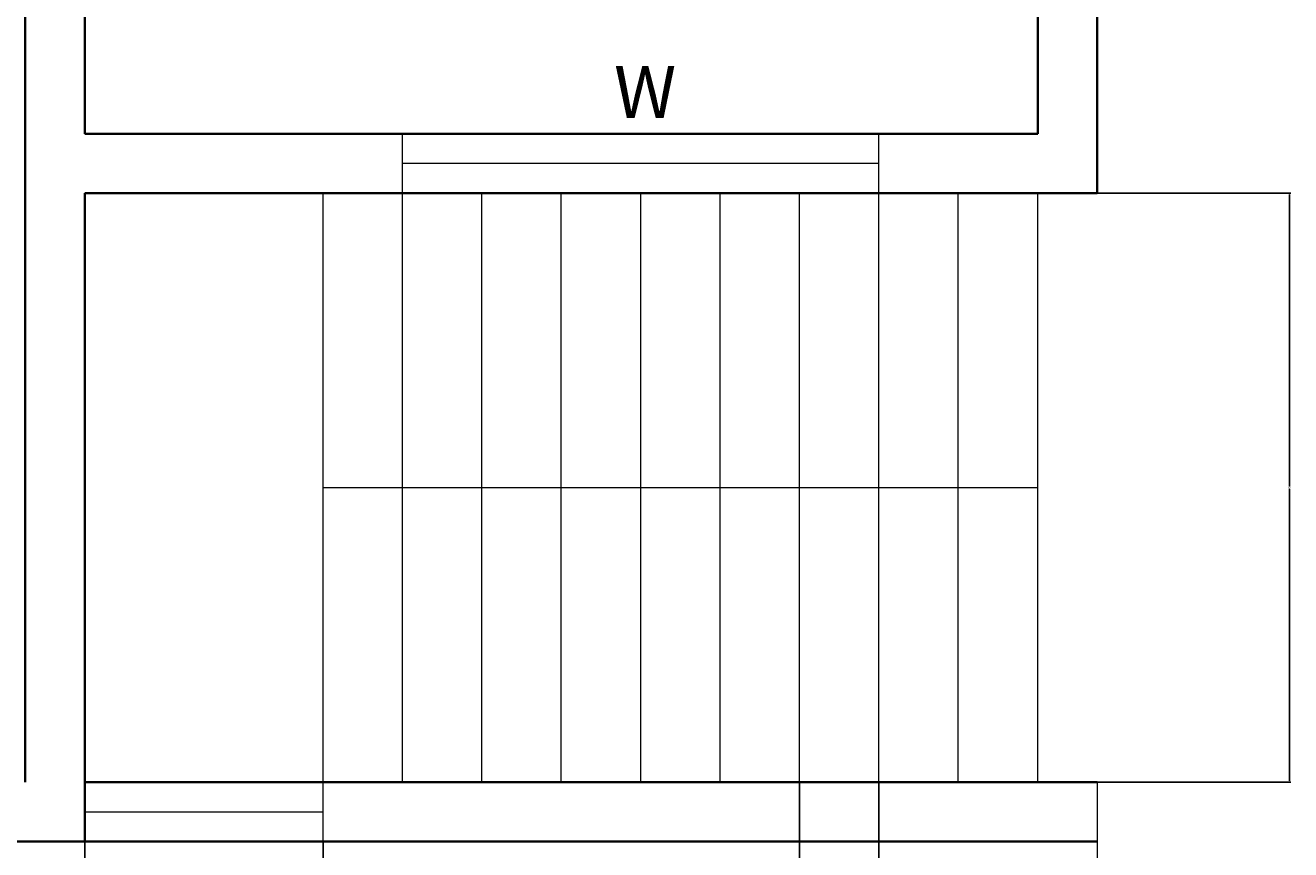
# Model space of a CAD drawing. Units: feet. Extents: x 2219 to 3039, y 1768 to 2369.
# Tile 4 of 16: x 2601 to 2793, y 1897 to 2021. Entities that reach past the tile are written whole.
import ezdxf

# ---------------------------------------------------------------- set-up
doc = ezdxf.new("R2010")
doc.units = ezdxf.units.FT
for name, color, linetype, lineweight in [('A-ANNO-DIMS', 2, 'Continuous', 18), ('A-ANNO-TEXT', 7, 'Continuous', 18), ('A-FLOR-STRS', 7, 'Continuous', 18), ('A-GLAZ', 4, 'Continuous', 18), ('A-WALL', 7, 'Continuous', 35), ('C-SITE', 3, 'Continuous', 20)]:
    doc.layers.add(name, color=color, linetype=linetype, lineweight=lineweight)
doc.styles.get("Standard").update_dxf_attribs({"font": 'arial.ttf'})
doc.dimstyles.get("Standard").update_dxf_attribs({"dimtxt": 0.18, "dimasz": 0.18, "dimexe": 0.18, "dimexo": 0.0625, "dimgap": 0.09, "dimtad": 0, "dimtih": 1, "dimtoh": 1, "dimdec": 4, "dimzin": 0, "dimdsep": 46, "dimtxsty": 'Standard', "dimcen": 0.09, "dimadec": 0, "dimazin": 0, "dimtfac": 1, "dimtdec": 4, "dimtofl": 0, "dimtmove": 0, "dimatfit": 3, "dimfxl": 1, "dimtolj": 1, "dimtzin": 0, "dimarcsym": 0})

# ---------------------------------------------------------------- blocks, each defined once
blk = doc.blocks.new('*D61')
at = {"layer": 'A-ANNO-DIMS', "color": 0, "lineweight": -2, "transparency": 16777216}
for p, q in [((2754.46, 1995.92), (2792.63, 1995.92)), ((2792.45, 1995.74), (2792.45, 1951.6)), ((2792.45, 1907.1), (2792.45, 1951.24)), ((2754.46, 1906.92), (2792.63, 1906.92))]:
    blk.add_line(p, q, dxfattribs=at)
at = {"layer": 'A-ANNO-DIMS', "color": 0, "transparency": 16777216}
for points in [[(2792.42, 1995.74), (2792.48, 1995.74), (2792.45, 1995.92)], [(2792.42, 1907.1), (2792.48, 1907.1), (2792.45, 1906.92)]]:
    blk.add_solid(points, dxfattribs=at)
at = {"layer": 'Defpoints', "color": 0, "transparency": 16777216}
for p in [(2754.4, 1995.92), (2754.4, 1906.92), (2792.45, 1906.92)]:
    blk.add_point(p, dxfattribs=at)
at = {"layer": 'A-ANNO-DIMS', "color": 0, "transparency": 16777216, "insert": (2792.45, 1951.42), "char_height": 0.18, "attachment_point": 5}
blk.add_mtext('\\A1;89', dxfattribs=at)
blk = doc.blocks.new('*D62')
at = {"layer": 'A-ANNO-DIMS', "color": 0, "lineweight": -2, "transparency": 16777216}
for p, q in [((2610.4, 1897.86), (2610.4, 1859.69)), ((2646.4, 1897.86), (2646.4, 1859.69)), ((2610.58, 1859.87), (2628.18, 1859.87)), ((2646.22, 1859.87), (2628.62, 1859.87))]:
    blk.add_line(p, q, dxfattribs=at)
at = {"layer": 'A-ANNO-DIMS', "color": 0, "transparency": 16777216}
for points in [[(2610.58, 1859.9), (2610.58, 1859.84), (2610.4, 1859.87)], [(2646.22, 1859.9), (2646.22, 1859.84), (2646.4, 1859.87)]]:
    blk.add_solid(points, dxfattribs=at)
at = {"layer": 'Defpoints', "color": 0, "transparency": 16777216}
for p in [(2610.4, 1897.92), (2646.4, 1897.92), (2610.4, 1859.87)]:
    blk.add_point(p, dxfattribs=at)
at = {"layer": 'A-ANNO-DIMS', "color": 0, "transparency": 16777216, "insert": (2628.4, 1859.87), "char_height": 0.18, "attachment_point": 5}
blk.add_mtext('\\A1;36', dxfattribs=at)
blk = doc.blocks.new('*D63')
at = {"layer": 'A-ANNO-DIMS', "color": 0, "lineweight": -2, "transparency": 16777216}
for p, q in [((2718.4, 1906.86), (2718.4, 1868.69)), ((2730.4, 1906.86), (2730.4, 1868.69)), ((2718.58, 1868.87), (2724.19, 1868.87)), ((2730.22, 1868.87), (2724.61, 1868.87))]:
    blk.add_line(p, q, dxfattribs=at)
at = {"layer": 'A-ANNO-DIMS', "color": 0, "transparency": 16777216}
for points in [[(2718.58, 1868.9), (2718.58, 1868.84), (2718.4, 1868.87)], [(2730.22, 1868.9), (2730.22, 1868.84), (2730.4, 1868.87)]]:
    blk.add_solid(points, dxfattribs=at)
at = {"layer": 'Defpoints', "color": 0, "transparency": 16777216}
for p in [(2718.4, 1906.92), (2730.4, 1906.92), (2718.4, 1868.87)]:
    blk.add_point(p, dxfattribs=at)
at = {"layer": 'A-ANNO-DIMS', "color": 0, "transparency": 16777216, "insert": (2724.4, 1868.87), "char_height": 0.18, "attachment_point": 5}
blk.add_mtext('\\A1;12', dxfattribs=at)

msp = doc.modelspace()

# ---------------------------------------------------------------- linework, layer by layer
at = {"layer": 'A-FLOR-STRS'}
for p, q in [((2658.4, 1906.923), (2658.4, 2004.923)), ((2730.4, 1906.923), (2730.4, 2004.923)), ((2646.4, 1897.923), (2646.4, 1995.923)), ((2670.4, 1906.923), (2670.4, 1995.923)), ((2682.4, 1906.923), (2682.4, 1995.923)), ((2694.4, 1906.923), (2694.4, 1995.923)), ((2706.4, 1906.923), (2706.4, 1995.923)), ((2718.4, 1906.923), (2718.4, 1995.923)), ((2742.4, 1906.923), (2742.4, 1995.923)), ((2754.4, 1906.923), (2754.4, 1995.923)), ((2646.4, 1951.423), (2754.4, 1951.423))]:
    msp.add_line(p, q, dxfattribs=at)
at = {"layer": 'A-GLAZ'}
for p, q in [((2730.4, 2000.423), (2658.4, 2000.423)), ((2610.4, 1902.423), (2646.4, 1902.423))]:
    msp.add_line(p, q, dxfattribs=at)
at = {"layer": 'A-WALL'}
for p, q in [((2610.4, 2004.923), (2610.4, 2112.923)), ((2754.4, 2085.923), (2754.4, 2004.923)), ((2763.4, 2085.923), (2763.4, 1995.923)), ((2601.4, 1906.923), (2601.4, 2058.923)), ((2754.4, 2004.923), (2610.4, 2004.923)), ((2610.4, 1897.923), (2610.4, 1995.923)), ((2763.4, 1995.923), (2610.4, 1995.923)), ((2610.4, 1906.923), (2763.4, 1906.923)), ((2610.4, 1897.923), (2443.4, 1897.923)), ((2605.4, 1897.923), (2610.4, 1897.923)), ((2610.4, 1897.923), (2763.4, 1897.923))]:
    msp.add_line(p, q, dxfattribs=at)
at = {"layer": 'C-SITE'}
msp.add_line((2763.4, 1906.923), (2763.4, 1828.923), dxfattribs=at)

# ---------------------------------------------------------------- texts
at = {"layer": 'A-ANNO-TEXT'}
msp.add_text('W', height=7.858, dxfattribs=at).set_placement((2690.362, 2007.308))

# ---------------------------------------------------------------- dimensions: what is measured, and where the dimension line sits
at = {"layer": 'A-ANNO-DIMS'}
for base, p1, p2, angle, picture, middle in [((2792.45, 1906.923), (2754.4, 1995.923), (2754.4, 1906.923), 270, '*D61', (2792.45, 1951.423)), ((2718.4, 1868.873), (2730.4, 1906.923), (2718.4, 1906.923), 180, '*D63', (2724.4, 1868.873)), ((2610.4, 1859.873), (2646.4, 1897.923), (2610.4, 1897.923), 180, '*D62', (2628.4, 1859.873))]:
    dim = msp.add_linear_dim(base=base, p1=p1, p2=p2, angle=angle, dimstyle='Standard', override={"dimdec": 0, "dimlfac": 1, "dimrnd": 0, "dimzin": 0, "dimdsep": 46, "dimlunit": 2}, dxfattribs=at)
    dim.commit()
    dim.dimension.update_dxf_attribs({"geometry": picture, "text_midpoint": middle})

doc.saveas('drawing.dxf')
